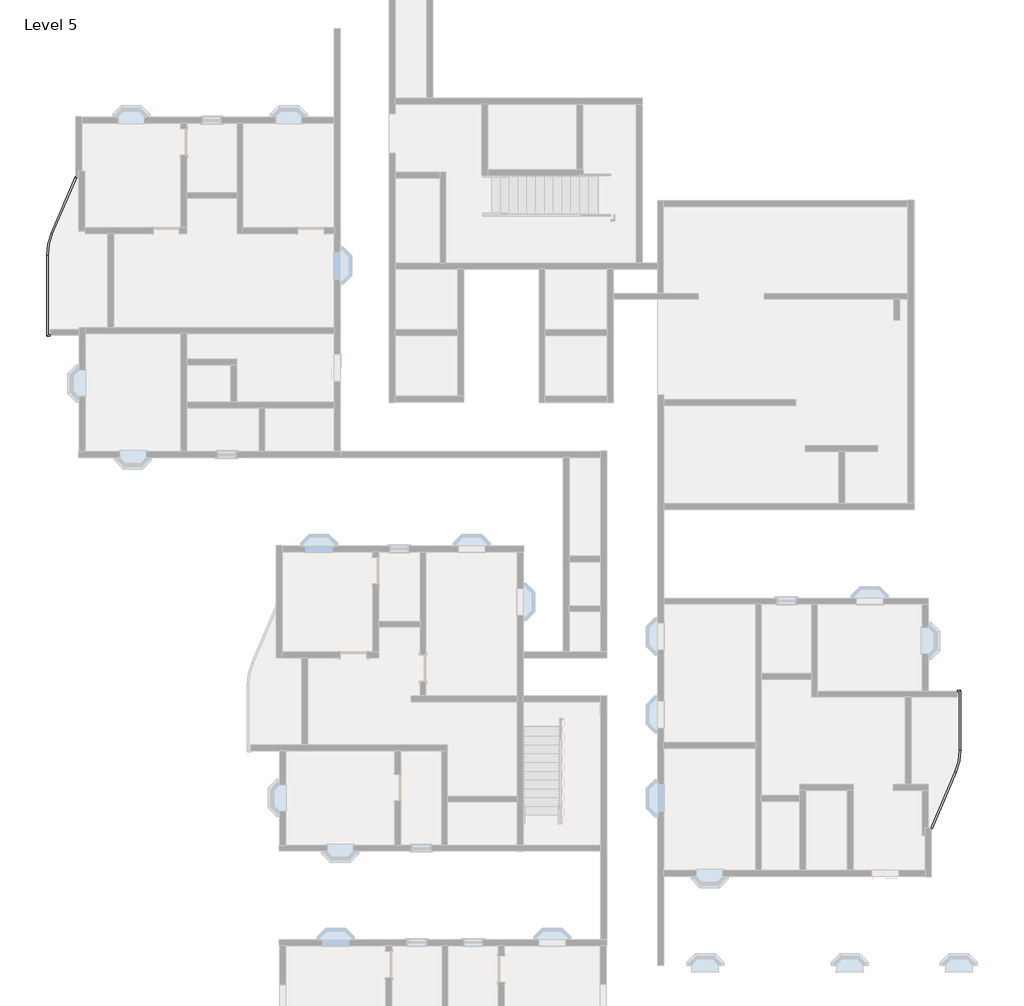
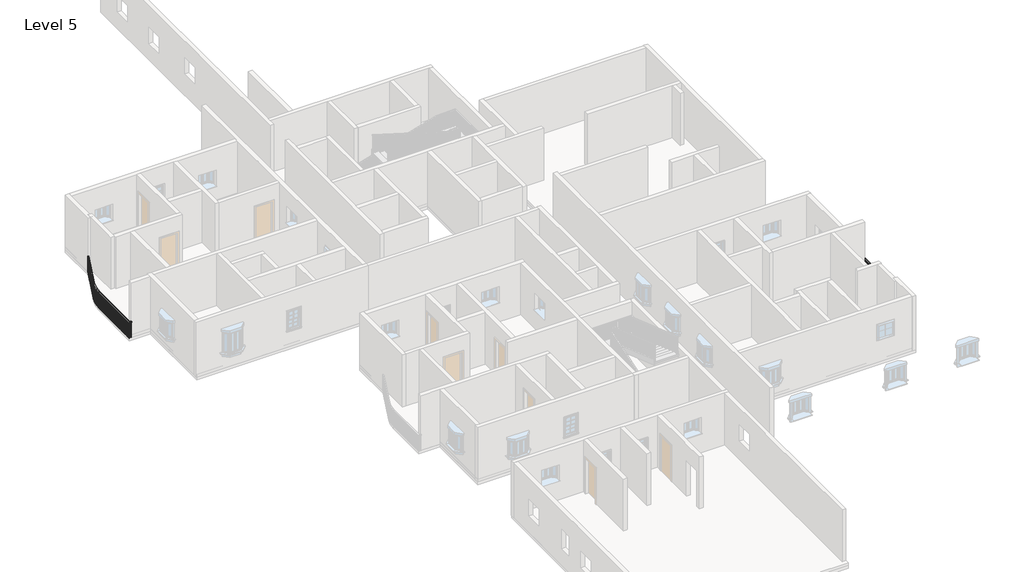
# One storey, part 9 of 14: 2 railings.
"""IFC4 building model written with IfcOpenShell, lengths in millimetres."""

from ifc_helpers import new_model, si_unit, frame, origin, place, context, project, spatial, polyline, circle_curve, outline, extrude, element, save
from ifc_brep_helpers import plane_surface, cylinder_surface, revolved_surface, advanced_brep

model = new_model("IFC4")

# Units and contexts
model_context = context("Model", 3, world=origin())
ifc_project = project(units=[si_unit("LENGTHUNIT", "METRE", prefix="MILLI")], contexts=[model_context])

# Site, building, storey
site = spatial("IfcSite", under=ifc_project)
building = spatial("IfcBuilding", under=site)
storey = spatial("IfcBuildingStorey", under=building, Name="Level 5", Elevation=12192.0)

# Railings
placement = place(None, origin())
element("IfcRailing", 1, ObjectType="Handrail - Rectangular", at=placement, inside=storey, context=model_context, shape_type="SolidModel", body=[
    advanced_brep(
    [(-19327.739878, 12446.0257339, 13106.4), (-19327.739878, 12446.0257339, 13055.6), (-19374.4383922, 12466.022953, 13055.6), (-19374.4383922, 12466.022953, 13106.4), (-20162.483418, 10496.6905323, 13106.4), (-20162.483418, 10496.6905323, 13055.6), (-20209.1819322, 10516.6877514, 13055.6), (-20209.1819322, 10516.6877514, 13106.4), (-20316.2891351, 9746.7948172, 13055.6), (-20316.2891351, 9746.7948172, 13106.4), (-20367.0891351, 9746.7948172, 13055.6), (-20367.0891351, 9746.7948172, 13106.4), (-20316.2891351, 7005.2583494, 13106.4), (-20316.2891351, 7005.2583494, 13055.6), (-20367.0891351, 6954.4583494, 13055.6), (-20367.0891351, 6954.4583494, 13106.4), (-20240.0891351, 7005.2583494, 13106.4), (-20240.0891351, 6954.4583494, 13106.4), (-20240.0891351, 6954.4583494, 13055.6), (-20240.0891351, 7005.2583494, 13055.6)],
    [
        (0, 1),
        (1, 2),
        (2, 3),
        (3, 0),
        (0, 4),
        (4, 5),
        (5, 1),
        (5, 6),
        (6, 2),
        (6, 7),
        (7, 3),
        (7, 4),
        (8, 5, circle_curve(frame((-18411.2891351, 9746.7948172, 13055.6), z_axis=(0.0, 0.0, -1.0), x_axis=(-0.919262090762392, 0.3936460446735823, 0.0)), 1905.0)),
        (4, 9, circle_curve(frame((-18411.2891351, 9746.7948172, 13106.4), z_axis=(0.0, 0.0, 1.0), x_axis=(-0.919262090762392, 0.3936460446735823, 0.0)), 1905.0)),
        (9, 8),
        (10, 6, circle_curve(frame((-18411.2891351, 9746.7948172, 13055.6), z_axis=(0.0, 0.0, -1.0), x_axis=(-0.919262090762392, 0.3936460446735823, 0.0)), 1955.8)),
        (8, 10),
        (11, 7, circle_curve(frame((-18411.2891351, 9746.7948172, 13106.4), z_axis=(0.0, 0.0, -1.0), x_axis=(-0.919262090762392, 0.3936460446735823, 0.0)), 1955.8)),
        (10, 11),
        (11, 9),
        (9, 12),
        (12, 13),
        (13, 8),
        (13, 14),
        (14, 10),
        (14, 15),
        (15, 11),
        (15, 12),
        (16, 17),
        (17, 18),
        (18, 19),
        (19, 16),
        (12, 16),
        (19, 13),
        (18, 14),
        (17, 15),
    ],
    [
        plane_surface(frame((-19351.0891351, 12456.0243434, 13106.4), z_axis=(0.3936460446735829, 0.9192620907623917, 0.0), x_axis=(0.9192620907623917, -0.3936460446735829, 0.0))),
        plane_surface(frame((-19327.739878, 12446.0257339, 13106.4), z_axis=(0.9192620907623915, -0.3936460446735834, 0.0), x_axis=(-0.3936460446735834, -0.9192620907623915, 0.0))),
        plane_surface(frame((-19327.739878, 12446.0257339, 13055.6), z_axis=(0.0, 0.0, -1.0000000000000002), x_axis=(-0.3936460446735834, -0.9192620907623915, 0.0))),
        plane_surface(frame((-19374.4383922, 12466.022953, 13055.6), z_axis=(-0.9192620907623916, 0.393646044673583, 0.0), x_axis=(-0.393646044673583, -0.9192620907623916, 0.0))),
        plane_surface(frame((-19374.4383922, 12466.022953, 13106.4), z_axis=(0.0, 0.0, 1.0), x_axis=(-0.393646044673583, -0.9192620907623916, 0.0))),
        revolved_surface(polyline([(-20162.483418002357, 10496.690532303173, 13106.4), (-20162.483418002357, 10496.690532303173, 13055.6)]), (-18411.2891351, 9746.7948172, 13106.4), (0.0, 0.0, 1.0)),
        plane_surface(frame((-18411.2891351, 9746.7948172, 13055.6), z_axis=(0.0, 0.0, -1.0), x_axis=(-0.919262090762392, 0.3936460446735823, 0.0))),
        cylinder_surface(frame((-18411.2891351, 9746.7948172, 13106.4), z_axis=(0.0, 0.0, 1.0), x_axis=(-0.919262090762392, 0.3936460446735823, 0.0)), 1955.8),
        plane_surface(frame((-18411.2891351, 9746.7948172, 13106.4), z_axis=(0.0, 0.0, 1.0), x_axis=(-0.919262090762392, 0.3936460446735823, 0.0))),
        plane_surface(frame((-20316.2891351, 9746.7948172, 13106.4), z_axis=(1.0, 0.0, 0.0), x_axis=(0.0, -1.0, 0.0))),
        plane_surface(frame((-20316.2891351, 9746.7948172, 13055.6), z_axis=(0.0, 0.0, -1.0), x_axis=(0.0, -1.0, 0.0))),
        plane_surface(frame((-20367.0891351, 9746.7948172, 13055.6), z_axis=(-1.0, 0.0, 0.0), x_axis=(0.0, -1.0, 0.0))),
        plane_surface(frame((-20367.0891351, 9746.7948172, 13106.4), z_axis=(0.0, 0.0, 1.0), x_axis=(0.0, -1.0, 0.0))),
        plane_surface(frame((-20240.0891351, 6979.8583494, 13106.4), z_axis=(1.0, 0.0, 0.0), x_axis=(0.0, 1.0, 0.0))),
        plane_surface(frame((-20316.2891351, 7005.2583494, 13106.4), z_axis=(0.0, 1.0, 0.0), x_axis=(1.0, 0.0, 0.0))),
        plane_surface(frame((-20316.2891351, 7005.2583494, 13055.6), z_axis=(0.0, 0.0, -1.0), x_axis=(1.0, 0.0, 0.0))),
        plane_surface(frame((-20367.0891351, 6954.4583494, 13055.6), z_axis=(0.0, -1.0, 0.0), x_axis=(1.0, 0.0, 0.0))),
        plane_surface(frame((-20367.0891351, 6954.4583494, 13106.4), z_axis=(0.0, 0.0, 1.0), x_axis=(1.0, 0.0, 0.0))),
    ],
    [
        (0, [[1, 2, 3, 4]]),
        (1, [[-1, 5, 6, 7]]),
        (2, [[-2, -7, 8, 9]]),
        (3, [[-3, -9, 10, 11]]),
        (4, [[-4, -11, 12, -5]]),
        (5, [[13, -6, 14, 15]]),
        (6, [[16, -8, -13, 17]]),
        (7, [[18, -10, -16, 19]]),
        (8, [[-14, -12, -18, 20]]),
        (9, [[-15, 21, 22, 23]]),
        (10, [[-17, -23, 24, 25]]),
        (11, [[-19, -25, 26, 27]]),
        (12, [[-20, -27, 28, -21]]),
        (13, [[29, 30, 31, 32]]),
        (14, [[-22, 33, -32, 34]]),
        (15, [[-24, -34, -31, 35]]),
        (16, [[-26, -35, -30, 36]]),
        (17, [[-28, -36, -29, -33]]),
    ],
),
    extrude(outline(polyline([(-20351.2141351, 7013.1198172), (-20332.1641351, 7013.1198172), (-20332.1641351, 6994.0698172), (-20351.2141351, 6994.0698172), (-20351.2141351, 7013.1198172)])), frame((0.0, 0.0, 12192.0), z_axis=(0.0, 0.0, 1.0), x_axis=(1.0, 0.0, 0.0)), (0.0, 0.0, 1.0), 863.6),
    extrude(outline(polyline([(-20351.2141351, 7114.7198172), (-20332.1641351, 7114.7198172), (-20332.1641351, 7095.6698172), (-20351.2141351, 7095.6698172), (-20351.2141351, 7114.7198172)])), frame((0.0, 0.0, 12192.0), z_axis=(0.0, 0.0, 1.0), x_axis=(1.0, 0.0, 0.0)), (0.0, 0.0, 1.0), 863.6),
    extrude(outline(polyline([(-20351.2141351, 7216.3198172), (-20332.1641351, 7216.3198172), (-20332.1641351, 7197.2698172), (-20351.2141351, 7197.2698172), (-20351.2141351, 7216.3198172)])), frame((0.0, 0.0, 12192.0), z_axis=(0.0, 0.0, 1.0), x_axis=(1.0, 0.0, 0.0)), (0.0, 0.0, 1.0), 863.6),
    extrude(outline(polyline([(-20351.2141351, 7317.9198172), (-20332.1641351, 7317.9198172), (-20332.1641351, 7298.8698172), (-20351.2141351, 7298.8698172), (-20351.2141351, 7317.9198172)])), frame((0.0, 0.0, 12192.0), z_axis=(0.0, 0.0, 1.0), x_axis=(1.0, 0.0, 0.0)), (0.0, 0.0, 1.0), 863.6),
    extrude(outline(polyline([(-20351.2141351, 7419.5198172), (-20332.1641351, 7419.5198172), (-20332.1641351, 7400.4698172), (-20351.2141351, 7400.4698172), (-20351.2141351, 7419.5198172)])), frame((0.0, 0.0, 12192.0), z_axis=(0.0, 0.0, 1.0), x_axis=(1.0, 0.0, 0.0)), (0.0, 0.0, 1.0), 863.6),
    extrude(outline(polyline([(-20351.2141351, 7521.1198172), (-20332.1641351, 7521.1198172), (-20332.1641351, 7502.0698172), (-20351.2141351, 7502.0698172), (-20351.2141351, 7521.1198172)])), frame((0.0, 0.0, 12192.0), z_axis=(0.0, 0.0, 1.0), x_axis=(1.0, 0.0, 0.0)), (0.0, 0.0, 1.0), 863.6),
    extrude(outline(polyline([(-20351.2141351, 7622.7198172), (-20332.1641351, 7622.7198172), (-20332.1641351, 7603.6698172), (-20351.2141351, 7603.6698172), (-20351.2141351, 7622.7198172)])), frame((0.0, 0.0, 12192.0), z_axis=(0.0, 0.0, 1.0), x_axis=(1.0, 0.0, 0.0)), (0.0, 0.0, 1.0), 863.6),
    extrude(outline(polyline([(-20351.2141351, 7724.3198172), (-20332.1641351, 7724.3198172), (-20332.1641351, 7705.2698172), (-20351.2141351, 7705.2698172), (-20351.2141351, 7724.3198172)])), frame((0.0, 0.0, 12192.0), z_axis=(0.0, 0.0, 1.0), x_axis=(1.0, 0.0, 0.0)), (0.0, 0.0, 1.0), 863.6),
    extrude(outline(polyline([(-20351.2141351, 7825.9198172), (-20332.1641351, 7825.9198172), (-20332.1641351, 7806.8698172), (-20351.2141351, 7806.8698172), (-20351.2141351, 7825.9198172)])), frame((0.0, 0.0, 12192.0), z_axis=(0.0, 0.0, 1.0), x_axis=(1.0, 0.0, 0.0)), (0.0, 0.0, 1.0), 863.6),
    extrude(outline(polyline([(-20351.2141351, 7927.5198172), (-20332.1641351, 7927.5198172), (-20332.1641351, 7908.4698172), (-20351.2141351, 7908.4698172), (-20351.2141351, 7927.5198172)])), frame((0.0, 0.0, 12192.0), z_axis=(0.0, 0.0, 1.0), x_axis=(1.0, 0.0, 0.0)), (0.0, 0.0, 1.0), 863.6),
    extrude(outline(polyline([(-20351.2141351, 8029.1198172), (-20332.1641351, 8029.1198172), (-20332.1641351, 8010.0698172), (-20351.2141351, 8010.0698172), (-20351.2141351, 8029.1198172)])), frame((0.0, 0.0, 12192.0), z_axis=(0.0, 0.0, 1.0), x_axis=(1.0, 0.0, 0.0)), (0.0, 0.0, 1.0), 863.6),
    extrude(outline(polyline([(-20351.2141351, 8130.7198172), (-20332.1641351, 8130.7198172), (-20332.1641351, 8111.6698172), (-20351.2141351, 8111.6698172), (-20351.2141351, 8130.7198172)])), frame((0.0, 0.0, 12192.0), z_axis=(0.0, 0.0, 1.0), x_axis=(1.0, 0.0, 0.0)), (0.0, 0.0, 1.0), 863.6),
    extrude(outline(polyline([(-20351.2141351, 8232.3198172), (-20332.1641351, 8232.3198172), (-20332.1641351, 8213.2698172), (-20351.2141351, 8213.2698172), (-20351.2141351, 8232.3198172)])), frame((0.0, 0.0, 12192.0), z_axis=(0.0, 0.0, 1.0), x_axis=(1.0, 0.0, 0.0)), (0.0, 0.0, 1.0), 863.6),
    extrude(outline(polyline([(-20351.2141351, 8333.9198172), (-20332.1641351, 8333.9198172), (-20332.1641351, 8314.8698172), (-20351.2141351, 8314.8698172), (-20351.2141351, 8333.9198172)])), frame((0.0, 0.0, 12192.0), z_axis=(0.0, 0.0, 1.0), x_axis=(1.0, 0.0, 0.0)), (0.0, 0.0, 1.0), 863.6),
    extrude(outline(polyline([(-20351.2141351, 8435.5198172), (-20332.1641351, 8435.5198172), (-20332.1641351, 8416.4698172), (-20351.2141351, 8416.4698172), (-20351.2141351, 8435.5198172)])), frame((0.0, 0.0, 12192.0), z_axis=(0.0, 0.0, 1.0), x_axis=(1.0, 0.0, 0.0)), (0.0, 0.0, 1.0), 863.6),
    extrude(outline(polyline([(-20351.2141351, 8537.1198172), (-20332.1641351, 8537.1198172), (-20332.1641351, 8518.0698172), (-20351.2141351, 8518.0698172), (-20351.2141351, 8537.1198172)])), frame((0.0, 0.0, 12192.0), z_axis=(0.0, 0.0, 1.0), x_axis=(1.0, 0.0, 0.0)), (0.0, 0.0, 1.0), 863.6),
    extrude(outline(polyline([(-20351.2141351, 8638.7198172), (-20332.1641351, 8638.7198172), (-20332.1641351, 8619.6698172), (-20351.2141351, 8619.6698172), (-20351.2141351, 8638.7198172)])), frame((0.0, 0.0, 12192.0), z_axis=(0.0, 0.0, 1.0), x_axis=(1.0, 0.0, 0.0)), (0.0, 0.0, 1.0), 863.6),
    extrude(outline(polyline([(-20351.2141351, 8740.3198172), (-20332.1641351, 8740.3198172), (-20332.1641351, 8721.2698172), (-20351.2141351, 8721.2698172), (-20351.2141351, 8740.3198172)])), frame((0.0, 0.0, 12192.0), z_axis=(0.0, 0.0, 1.0), x_axis=(1.0, 0.0, 0.0)), (0.0, 0.0, 1.0), 863.6),
    extrude(outline(polyline([(-20351.2141351, 8841.9198172), (-20332.1641351, 8841.9198172), (-20332.1641351, 8822.8698172), (-20351.2141351, 8822.8698172), (-20351.2141351, 8841.9198172)])), frame((0.0, 0.0, 12192.0), z_axis=(0.0, 0.0, 1.0), x_axis=(1.0, 0.0, 0.0)), (0.0, 0.0, 1.0), 863.6),
    extrude(outline(polyline([(-20351.2141351, 8943.5198172), (-20332.1641351, 8943.5198172), (-20332.1641351, 8924.4698172), (-20351.2141351, 8924.4698172), (-20351.2141351, 8943.5198172)])), frame((0.0, 0.0, 12192.0), z_axis=(0.0, 0.0, 1.0), x_axis=(1.0, 0.0, 0.0)), (0.0, 0.0, 1.0), 863.6),
    extrude(outline(polyline([(-20351.2141351, 9045.1198172), (-20332.1641351, 9045.1198172), (-20332.1641351, 9026.0698172), (-20351.2141351, 9026.0698172), (-20351.2141351, 9045.1198172)])), frame((0.0, 0.0, 12192.0), z_axis=(0.0, 0.0, 1.0), x_axis=(1.0, 0.0, 0.0)), (0.0, 0.0, 1.0), 863.6),
    extrude(outline(polyline([(-20351.2141351, 9146.7198172), (-20332.1641351, 9146.7198172), (-20332.1641351, 9127.6698172), (-20351.2141351, 9127.6698172), (-20351.2141351, 9146.7198172)])), frame((0.0, 0.0, 12192.0), z_axis=(0.0, 0.0, 1.0), x_axis=(1.0, 0.0, 0.0)), (0.0, 0.0, 1.0), 863.6),
    extrude(outline(polyline([(-20351.2141351, 9248.3198172), (-20332.1641351, 9248.3198172), (-20332.1641351, 9229.2698172), (-20351.2141351, 9229.2698172), (-20351.2141351, 9248.3198172)])), frame((0.0, 0.0, 12192.0), z_axis=(0.0, 0.0, 1.0), x_axis=(1.0, 0.0, 0.0)), (0.0, 0.0, 1.0), 863.6),
    extrude(outline(polyline([(-20351.2141351, 9349.9198172), (-20332.1641351, 9349.9198172), (-20332.1641351, 9330.8698172), (-20351.2141351, 9330.8698172), (-20351.2141351, 9349.9198172)])), frame((0.0, 0.0, 12192.0), z_axis=(0.0, 0.0, 1.0), x_axis=(1.0, 0.0, 0.0)), (0.0, 0.0, 1.0), 863.6),
    extrude(outline(polyline([(-20351.2141351, 9451.5198172), (-20332.1641351, 9451.5198172), (-20332.1641351, 9432.4698172), (-20351.2141351, 9432.4698172), (-20351.2141351, 9451.5198172)])), frame((0.0, 0.0, 12192.0), z_axis=(0.0, 0.0, 1.0), x_axis=(1.0, 0.0, 0.0)), (0.0, 0.0, 1.0), 863.6),
    extrude(outline(polyline([(-20351.2141351, 9553.1198172), (-20332.1641351, 9553.1198172), (-20332.1641351, 9534.0698172), (-20351.2141351, 9534.0698172), (-20351.2141351, 9553.1198172)])), frame((0.0, 0.0, 12192.0), z_axis=(0.0, 0.0, 1.0), x_axis=(1.0, 0.0, 0.0)), (0.0, 0.0, 1.0), 863.6),
    extrude(outline(polyline([(-20351.2141351, 9654.7198172), (-20332.1641351, 9654.7198172), (-20332.1641351, 9635.6698172), (-20351.2141351, 9635.6698172), (-20351.2141351, 9654.7198172)])), frame((0.0, 0.0, 12192.0), z_axis=(0.0, 0.0, 1.0), x_axis=(1.0, 0.0, 0.0)), (0.0, 0.0, 1.0), 863.6),
    extrude(outline(polyline([(-20349.6005818, 9826.4720848), (-20330.5630441, 9825.7831307), (-20331.2519982, 9806.745593), (-20350.289536, 9807.4345471), (-20349.6005818, 9826.4720848)])), frame((0.0, 0.0, 12192.0), z_axis=(0.0, 0.0, 1.0), x_axis=(1.0, 0.0, 0.0)), (0.0, 0.0, 1.0), 863.6),
    extrude(outline(polyline([(-20342.724955, 9928.3310534), (-20323.750023, 9926.6415402), (-20325.4395363, 9907.6666081), (-20344.4144683, 9909.3561214), (-20342.724955, 9928.3310534)])), frame((0.0, 0.0, 12192.0), z_axis=(0.0, 0.0, 1.0), x_axis=(1.0, 0.0, 0.0)), (0.0, 0.0, 1.0), 863.6),
    extrude(outline(polyline([(-20330.5003254, 10029.6872677), (-20311.6405491, 10027.0018743), (-20314.3259425, 10008.142098), (-20333.1857188, 10010.8274914), (-20330.5003254, 10029.6872677)])), frame((0.0, 0.0, 12192.0), z_axis=(0.0, 0.0, 1.0), x_axis=(1.0, 0.0, 0.0)), (0.0, 0.0, 1.0), 863.6),
    extrude(outline(polyline([(-20312.9605484, 10130.2600272), (-20294.2681589, 10126.5861907), (-20297.9419954, 10107.8938012), (-20316.6343849, 10111.5676377), (-20312.9605484, 10130.2600272)])), frame((0.0, 0.0, 12192.0), z_axis=(0.0, 0.0, 1.0), x_axis=(1.0, 0.0, 0.0)), (0.0, 0.0, 1.0), 863.6),
    extrude(outline(polyline([(-20290.1541995, 10229.7708014), (-20271.6809643, 10225.1186963), (-20276.3330693, 10206.6454611), (-20294.8063045, 10211.2975662), (-20290.1541995, 10229.7708014)])), frame((0.0, 0.0, 12192.0), z_axis=(0.0, 0.0, 1.0), x_axis=(1.0, 0.0, 0.0)), (0.0, 0.0, 1.0), 863.6),
    extrude(outline(polyline([(-20262.1444395, 10327.9440008), (-20243.9415192, 10322.3265109), (-20249.5590091, 10304.1235906), (-20267.7619294, 10309.7410805), (-20262.1444395, 10327.9440008)])), frame((0.0, 0.0, 12192.0), z_axis=(0.0, 0.0, 1.0), x_axis=(1.0, 0.0, 0.0)), (0.0, 0.0, 1.0), 863.6),
    extrude(outline(polyline([(-20229.0088399, 10424.5077402), (-20211.1266465, 10417.9404228), (-20217.693964, 10400.0582293), (-20235.5761574, 10406.6255468), (-20229.0088399, 10424.5077402)])), frame((0.0, 0.0, 12192.0), z_axis=(0.0, 0.0, 1.0), x_axis=(1.0, 0.0, 0.0)), (0.0, 0.0, 1.0), 863.6),
    extrude(outline(polyline([(-20155.9843907, 10600.589225), (-20138.4724479, 10593.0902678), (-20145.9714051, 10575.578325), (-20163.4833479, 10583.0772822), (-20155.9843907, 10600.589225)])), frame((0.0, 0.0, 12192.0), z_axis=(0.0, 0.0, 1.0), x_axis=(1.0, 0.0, 0.0)), (0.0, 0.0, 1.0), 863.6),
    extrude(outline(polyline([(-20115.9899526, 10693.9862534), (-20098.4780098, 10686.4872963), (-20105.9769669, 10668.9753534), (-20123.4889098, 10676.4743106), (-20115.9899526, 10693.9862534)])), frame((0.0, 0.0, 12192.0), z_axis=(0.0, 0.0, 1.0), x_axis=(1.0, 0.0, 0.0)), (0.0, 0.0, 1.0), 863.6),
    extrude(outline(polyline([(-20075.9955145, 10787.3832818), (-20058.4835716, 10779.8843247), (-20065.9825288, 10762.3723818), (-20083.4944716, 10769.871339), (-20075.9955145, 10787.3832818)])), frame((0.0, 0.0, 12192.0), z_axis=(0.0, 0.0, 1.0), x_axis=(1.0, 0.0, 0.0)), (0.0, 0.0, 1.0), 863.6),
    extrude(outline(polyline([(-20036.0010763, 10880.7803103), (-20018.4891335, 10873.2813531), (-20025.9880906, 10855.7694103), (-20043.5000335, 10863.2683674), (-20036.0010763, 10880.7803103)])), frame((0.0, 0.0, 12192.0), z_axis=(0.0, 0.0, 1.0), x_axis=(1.0, 0.0, 0.0)), (0.0, 0.0, 1.0), 863.6),
    extrude(outline(polyline([(-19996.0066382, 10974.1773387), (-19978.4946954, 10966.6783815), (-19985.9936525, 10949.1664387), (-20003.5055953, 10956.6653958), (-19996.0066382, 10974.1773387)])), frame((0.0, 0.0, 12192.0), z_axis=(0.0, 0.0, 1.0), x_axis=(1.0, 0.0, 0.0)), (0.0, 0.0, 1.0), 863.6),
    extrude(outline(polyline([(-19956.0122, 11067.5743671), (-19938.5002572, 11060.0754099), (-19945.9992144, 11042.5634671), (-19963.5111572, 11050.0624243), (-19956.0122, 11067.5743671)])), frame((0.0, 0.0, 12192.0), z_axis=(0.0, 0.0, 1.0), x_axis=(1.0, 0.0, 0.0)), (0.0, 0.0, 1.0), 863.6),
    extrude(outline(polyline([(-19916.0177619, 11160.9713955), (-19898.5058191, 11153.4724384), (-19906.0047762, 11135.9604955), (-19923.5167191, 11143.4594527), (-19916.0177619, 11160.9713955)])), frame((0.0, 0.0, 12192.0), z_axis=(0.0, 0.0, 1.0), x_axis=(1.0, 0.0, 0.0)), (0.0, 0.0, 1.0), 863.6),
    extrude(outline(polyline([(-19876.0233238, 11254.3684239), (-19858.5113809, 11246.8694668), (-19866.0103381, 11229.357524), (-19883.5222809, 11236.8564811), (-19876.0233238, 11254.3684239)])), frame((0.0, 0.0, 12192.0), z_axis=(0.0, 0.0, 1.0), x_axis=(1.0, 0.0, 0.0)), (0.0, 0.0, 1.0), 863.6),
    extrude(outline(polyline([(-19836.0288856, 11347.7654524), (-19818.5169428, 11340.2664952), (-19826.0159, 11322.7545524), (-19843.5278428, 11330.2535095), (-19836.0288856, 11347.7654524)])), frame((0.0, 0.0, 12192.0), z_axis=(0.0, 0.0, 1.0), x_axis=(1.0, 0.0, 0.0)), (0.0, 0.0, 1.0), 863.6),
    extrude(outline(polyline([(-19796.0344475, 11441.1624808), (-19778.5225047, 11433.6635236), (-19786.0214618, 11416.1515808), (-19803.5334046, 11423.650538), (-19796.0344475, 11441.1624808)])), frame((0.0, 0.0, 12192.0), z_axis=(0.0, 0.0, 1.0), x_axis=(1.0, 0.0, 0.0)), (0.0, 0.0, 1.0), 863.6),
    extrude(outline(polyline([(-19756.0400094, 11534.5595092), (-19738.5280665, 11527.060552), (-19746.0270237, 11509.5486092), (-19763.5389665, 11517.0475664), (-19756.0400094, 11534.5595092)])), frame((0.0, 0.0, 12192.0), z_axis=(0.0, 0.0, 1.0), x_axis=(1.0, 0.0, 0.0)), (0.0, 0.0, 1.0), 863.6),
    extrude(outline(polyline([(-19716.0455712, 11627.9565376), (-19698.5336284, 11620.4575805), (-19706.0325855, 11602.9456376), (-19723.5445284, 11610.4445948), (-19716.0455712, 11627.9565376)])), frame((0.0, 0.0, 12192.0), z_axis=(0.0, 0.0, 1.0), x_axis=(1.0, 0.0, 0.0)), (0.0, 0.0, 1.0), 863.6),
    extrude(outline(polyline([(-19676.0511331, 11721.353566), (-19658.5391902, 11713.8546089), (-19666.0381474, 11696.3426661), (-19683.5500902, 11703.8416232), (-19676.0511331, 11721.353566)])), frame((0.0, 0.0, 12192.0), z_axis=(0.0, 0.0, 1.0), x_axis=(1.0, 0.0, 0.0)), (0.0, 0.0, 1.0), 863.6),
    extrude(outline(polyline([(-19636.0566949, 11814.7505945), (-19618.5447521, 11807.2516373), (-19626.0437093, 11789.7396945), (-19643.5556521, 11797.2386516), (-19636.0566949, 11814.7505945)])), frame((0.0, 0.0, 12192.0), z_axis=(0.0, 0.0, 1.0), x_axis=(1.0, 0.0, 0.0)), (0.0, 0.0, 1.0), 863.6),
    extrude(outline(polyline([(-19596.0622568, 11908.1476229), (-19578.550314, 11900.6486657), (-19586.0492711, 11883.1367229), (-19603.561214, 11890.6356801), (-19596.0622568, 11908.1476229)])), frame((0.0, 0.0, 12192.0), z_axis=(0.0, 0.0, 1.0), x_axis=(1.0, 0.0, 0.0)), (0.0, 0.0, 1.0), 863.6),
    extrude(outline(polyline([(-19556.0678187, 12001.5446513), (-19538.5558758, 11994.0456942), (-19546.054833, 11976.5337513), (-19563.5667758, 11984.0327085), (-19556.0678187, 12001.5446513)])), frame((0.0, 0.0, 12192.0), z_axis=(0.0, 0.0, 1.0), x_axis=(1.0, 0.0, 0.0)), (0.0, 0.0, 1.0), 863.6),
    extrude(outline(polyline([(-19516.0733805, 12094.9416797), (-19498.5614377, 12087.4427226), (-19506.0603948, 12069.9307797), (-19523.5723377, 12077.4297369), (-19516.0733805, 12094.9416797)])), frame((0.0, 0.0, 12192.0), z_axis=(0.0, 0.0, 1.0), x_axis=(1.0, 0.0, 0.0)), (0.0, 0.0, 1.0), 863.6),
    extrude(outline(polyline([(-19476.0789424, 12188.3387082), (-19458.5669996, 12180.839751), (-19466.0659567, 12163.3278082), (-19483.5778995, 12170.8267653), (-19476.0789424, 12188.3387082)])), frame((0.0, 0.0, 12192.0), z_axis=(0.0, 0.0, 1.0), x_axis=(1.0, 0.0, 0.0)), (0.0, 0.0, 1.0), 863.6),
    extrude(outline(polyline([(-19436.0845042, 12281.7357366), (-19418.5725614, 12274.2367794), (-19426.0715186, 12256.7248366), (-19443.5834614, 12264.2237937), (-19436.0845042, 12281.7357366)])), frame((0.0, 0.0, 12192.0), z_axis=(0.0, 0.0, 1.0), x_axis=(1.0, 0.0, 0.0)), (0.0, 0.0, 1.0), 863.6),
    extrude(outline(polyline([(-19396.0900661, 12375.132765), (-19378.5781233, 12367.6338078), (-19386.0770804, 12350.121865), (-19403.5890233, 12357.6208222), (-19396.0900661, 12375.132765)])), frame((0.0, 0.0, 12192.0), z_axis=(0.0, 0.0, 1.0), x_axis=(1.0, 0.0, 0.0)), (0.0, 0.0, 1.0), 863.6),
    extrude(outline(polyline([(-20351.2141351, 6989.3833494), (-20332.1641351, 6989.3833494), (-20332.1641351, 6970.3333494), (-20351.2141351, 6970.3333494), (-20351.2141351, 6989.3833494)])), frame((0.0, 0.0, 12192.0), z_axis=(0.0, 0.0, 1.0), x_axis=(1.0, 0.0, 0.0)), (0.0, 0.0, 1.0), 863.6),
    extrude(outline(polyline([(-20351.2141351, 9756.3198172), (-20332.1641351, 9756.3198172), (-20332.1641351, 9737.2698172), (-20351.2141351, 9737.2698172), (-20351.2141351, 9756.3198172)])), frame((0.0, 0.0, 12192.0), z_axis=(0.0, 0.0, 1.0), x_axis=(1.0, 0.0, 0.0)), (0.0, 0.0, 1.0), 863.6),
    extrude(outline(polyline([(-20190.839168, 10519.1945919), (-20173.3272251, 10511.6956347), (-20180.8261823, 10494.1836919), (-20198.3381251, 10501.682649), (-20190.839168, 10519.1945919)])), frame((0.0, 0.0, 12192.0), z_axis=(0.0, 0.0, 1.0), x_axis=(1.0, 0.0, 0.0)), (0.0, 0.0, 1.0), 863.6),
    extrude(outline(polyline([(-20259.1391351, 6970.3333494), (-20259.1391351, 6989.3833494), (-20240.0891351, 6989.3833494), (-20240.0891351, 6970.3333494), (-20259.1391351, 6970.3333494)])), frame((0.0, 0.0, 12192.0), z_axis=(0.0, 0.0, 1.0), x_axis=(1.0, 0.0, 0.0)), (0.0, 0.0, 1.0), 863.6),
    extrude(outline(polyline([(-19359.8451065, 12459.773822), (-19342.3331637, 12452.2748648), (-19349.8321209, 12434.762922), (-19367.3440637, 12442.2618792), (-19359.8451065, 12459.773822)])), frame((0.0, 0.0, 12192.0), z_axis=(0.0, 0.0, 1.0), x_axis=(1.0, 0.0, 0.0)), (0.0, 0.0, 1.0), 863.6),
])
element("IfcRailing", 2, ObjectType="Handrail - Rectangular", at=placement, inside=storey, context=model_context, shape_type="SolidModel", body=[
    advanced_brep(
    [(10250.7887952, -10096.81198, 13106.4), (10250.7887952, -10096.81198, 13055.6), (10297.4873094, -10116.8091991, 13055.6), (10297.4873094, -10116.8091991, 13106.4), (11085.5323352, -8147.4767784, 13106.4), (11085.5323352, -8147.4767784, 13055.6), (11132.2308494, -8167.4739975, 13055.6), (11132.2308494, -8167.4739975, 13106.4), (11239.3380523, -7397.5810633, 13055.6), (11239.3380523, -7397.5810633, 13106.4), (11290.1380523, -7397.5810633, 13055.6), (11290.1380523, -7397.5810633, 13106.4), (11239.3380523, -5378.0542694, 13106.4), (11239.3380523, -5378.0542694, 13055.6), (11290.1380523, -5327.2542694, 13055.6), (11290.1380523, -5327.2542694, 13106.4), (11163.1380523, -5378.0542694, 13106.4), (11163.1380523, -5327.2542694, 13106.4), (11163.1380523, -5327.2542694, 13055.6), (11163.1380523, -5378.0542694, 13055.6)],
    [
        (0, 1),
        (1, 2),
        (2, 3),
        (3, 0),
        (0, 4),
        (4, 5),
        (5, 1),
        (5, 6),
        (6, 2),
        (6, 7),
        (7, 3),
        (7, 4),
        (8, 5, circle_curve(frame((9334.3380523, -7397.5810633, 13055.6), z_axis=(0.0, 0.0, -1.0), x_axis=(0.9192620907624003, -0.3936460446735628, 0.0)), 1905.0)),
        (4, 9, circle_curve(frame((9334.3380523, -7397.5810633, 13106.4), z_axis=(0.0, 0.0, 1.0), x_axis=(0.9192620907624003, -0.3936460446735628, 0.0)), 1905.0)),
        (9, 8),
        (10, 6, circle_curve(frame((9334.3380523, -7397.5810633, 13055.6), z_axis=(0.0, 0.0, -1.0), x_axis=(0.9192620907624003, -0.3936460446735628, 0.0)), 1955.8)),
        (8, 10),
        (11, 7, circle_curve(frame((9334.3380523, -7397.5810633, 13106.4), z_axis=(0.0, 0.0, -1.0), x_axis=(0.9192620907624003, -0.3936460446735628, 0.0)), 1955.8)),
        (10, 11),
        (11, 9),
        (9, 12),
        (12, 13),
        (13, 8),
        (13, 14),
        (14, 10),
        (14, 15),
        (15, 11),
        (15, 12),
        (16, 17),
        (17, 18),
        (18, 19),
        (19, 16),
        (12, 16),
        (19, 13),
        (18, 14),
        (17, 15),
    ],
    [
        plane_surface(frame((10274.1380523, -10106.8105895, 13106.4), z_axis=(-0.3936460446735629, -0.9192620907624003, 0.0), x_axis=(0.9192620907624003, -0.3936460446735629, 0.0))),
        plane_surface(frame((10250.7887952, -10096.81198, 13106.4), z_axis=(-0.9192620907624005, 0.39364604467356235, 0.0), x_axis=(0.39364604467356235, 0.9192620907624005, 0.0))),
        plane_surface(frame((10250.7887952, -10096.81198, 13055.6), z_axis=(0.0, 0.0, -1.0), x_axis=(0.39364604467356235, 0.9192620907624005, 0.0))),
        plane_surface(frame((10297.4873094, -10116.8091991, 13055.6), z_axis=(0.9192620907624003, -0.3936460446735627, 0.0), x_axis=(0.3936460446735627, 0.9192620907624003, 0.0))),
        plane_surface(frame((10297.4873094, -10116.8091991, 13106.4), z_axis=(0.0, 0.0, 1.0), x_axis=(0.3936460446735627, 0.9192620907624003, 0.0))),
        revolved_surface(polyline([(11085.532335202372, -8147.476778403137, 13106.4), (11085.532335202372, -8147.476778403137, 13055.6)]), (9334.3380523, -7397.5810633, 13106.4), (0.0, 0.0, 1.0)),
        plane_surface(frame((9334.3380523, -7397.5810633, 13055.6), z_axis=(0.0, 0.0, -1.0), x_axis=(0.9192620907624003, -0.3936460446735628, 0.0))),
        cylinder_surface(frame((9334.3380523, -7397.5810633, 13106.4), z_axis=(0.0, 0.0, 1.0), x_axis=(0.9192620907624003, -0.3936460446735628, 0.0)), 1955.8),
        plane_surface(frame((9334.3380523, -7397.5810633, 13106.4), z_axis=(0.0, 0.0, 1.0), x_axis=(0.9192620907624003, -0.3936460446735628, 0.0))),
        plane_surface(frame((11239.3380523, -7397.5810633, 13106.4), z_axis=(-1.0, 0.0, 0.0), x_axis=(0.0, 1.0, 0.0))),
        plane_surface(frame((11239.3380523, -7397.5810633, 13055.6), z_axis=(0.0, 0.0, -1.0), x_axis=(0.0, 1.0, 0.0))),
        plane_surface(frame((11290.1380523, -7397.5810633, 13055.6), z_axis=(1.0, 0.0, 0.0), x_axis=(0.0, 1.0, 0.0))),
        plane_surface(frame((11290.1380523, -7397.5810633, 13106.4), z_axis=(0.0, 0.0, 1.0), x_axis=(0.0, 1.0, 0.0))),
        plane_surface(frame((11163.1380523, -5352.6542694, 13106.4), z_axis=(-1.0, 0.0, 0.0), x_axis=(0.0, -1.0, 0.0))),
        plane_surface(frame((11239.3380523, -5378.0542694, 13106.4), z_axis=(0.0, -1.0, 0.0), x_axis=(-1.0, 0.0, 0.0))),
        plane_surface(frame((11239.3380523, -5378.0542694, 13055.6), z_axis=(0.0, 0.0, -1.0), x_axis=(-1.0, 0.0, 0.0))),
        plane_surface(frame((11290.1380523, -5327.2542694, 13055.6), z_axis=(0.0, 1.0, 0.0), x_axis=(-1.0, 0.0, 0.0))),
        plane_surface(frame((11290.1380523, -5327.2542694, 13106.4), z_axis=(0.0, 0.0, 1.0), x_axis=(-1.0, 0.0, 0.0))),
    ],
    [
        (0, [[1, 2, 3, 4]]),
        (1, [[-1, 5, 6, 7]]),
        (2, [[-2, -7, 8, 9]]),
        (3, [[-3, -9, 10, 11]]),
        (4, [[-4, -11, 12, -5]]),
        (5, [[13, -6, 14, 15]]),
        (6, [[16, -8, -13, 17]]),
        (7, [[18, -10, -16, 19]]),
        (8, [[-14, -12, -18, 20]]),
        (9, [[-15, 21, 22, 23]]),
        (10, [[-17, -23, 24, 25]]),
        (11, [[-19, -25, 26, 27]]),
        (12, [[-20, -27, 28, -21]]),
        (13, [[29, 30, 31, 32]]),
        (14, [[-22, 33, -32, 34]]),
        (15, [[-24, -34, -31, 35]]),
        (16, [[-26, -35, -30, 36]]),
        (17, [[-28, -36, -29, -33]]),
    ],
),
    extrude(outline(polyline([(11274.2630523, -5375.1060633), (11255.2130523, -5375.1060633), (11255.2130523, -5356.0560633), (11274.2630523, -5356.0560633), (11274.2630523, -5375.1060633)])), frame((0.0, 0.0, 12192.0), z_axis=(0.0, 0.0, 1.0), x_axis=(1.0, 0.0, 0.0)), (0.0, 0.0, 1.0), 863.6),
    extrude(outline(polyline([(11274.2630523, -5476.7060633), (11255.2130523, -5476.7060633), (11255.2130523, -5457.6560633), (11274.2630523, -5457.6560633), (11274.2630523, -5476.7060633)])), frame((0.0, 0.0, 12192.0), z_axis=(0.0, 0.0, 1.0), x_axis=(1.0, 0.0, 0.0)), (0.0, 0.0, 1.0), 863.6),
    extrude(outline(polyline([(11274.2630523, -5578.3060633), (11255.2130523, -5578.3060633), (11255.2130523, -5559.2560633), (11274.2630523, -5559.2560633), (11274.2630523, -5578.3060633)])), frame((0.0, 0.0, 12192.0), z_axis=(0.0, 0.0, 1.0), x_axis=(1.0, 0.0, 0.0)), (0.0, 0.0, 1.0), 863.6),
    extrude(outline(polyline([(11274.2630523, -5679.9060633), (11255.2130523, -5679.9060633), (11255.2130523, -5660.8560633), (11274.2630523, -5660.8560633), (11274.2630523, -5679.9060633)])), frame((0.0, 0.0, 12192.0), z_axis=(0.0, 0.0, 1.0), x_axis=(1.0, 0.0, 0.0)), (0.0, 0.0, 1.0), 863.6),
    extrude(outline(polyline([(11274.2630523, -5781.5060633), (11255.2130523, -5781.5060633), (11255.2130523, -5762.4560633), (11274.2630523, -5762.4560633), (11274.2630523, -5781.5060633)])), frame((0.0, 0.0, 12192.0), z_axis=(0.0, 0.0, 1.0), x_axis=(1.0, 0.0, 0.0)), (0.0, 0.0, 1.0), 863.6),
    extrude(outline(polyline([(11274.2630523, -5883.1060633), (11255.2130523, -5883.1060633), (11255.2130523, -5864.0560633), (11274.2630523, -5864.0560633), (11274.2630523, -5883.1060633)])), frame((0.0, 0.0, 12192.0), z_axis=(0.0, 0.0, 1.0), x_axis=(1.0, 0.0, 0.0)), (0.0, 0.0, 1.0), 863.6),
    extrude(outline(polyline([(11274.2630523, -5984.7060633), (11255.2130523, -5984.7060633), (11255.2130523, -5965.6560633), (11274.2630523, -5965.6560633), (11274.2630523, -5984.7060633)])), frame((0.0, 0.0, 12192.0), z_axis=(0.0, 0.0, 1.0), x_axis=(1.0, 0.0, 0.0)), (0.0, 0.0, 1.0), 863.6),
    extrude(outline(polyline([(11274.2630523, -6086.3060633), (11255.2130523, -6086.3060633), (11255.2130523, -6067.2560633), (11274.2630523, -6067.2560633), (11274.2630523, -6086.3060633)])), frame((0.0, 0.0, 12192.0), z_axis=(0.0, 0.0, 1.0), x_axis=(1.0, 0.0, 0.0)), (0.0, 0.0, 1.0), 863.6),
    extrude(outline(polyline([(11274.2630523, -6187.9060633), (11255.2130523, -6187.9060633), (11255.2130523, -6168.8560633), (11274.2630523, -6168.8560633), (11274.2630523, -6187.9060633)])), frame((0.0, 0.0, 12192.0), z_axis=(0.0, 0.0, 1.0), x_axis=(1.0, 0.0, 0.0)), (0.0, 0.0, 1.0), 863.6),
    extrude(outline(polyline([(11274.2630523, -6289.5060633), (11255.2130523, -6289.5060633), (11255.2130523, -6270.4560633), (11274.2630523, -6270.4560633), (11274.2630523, -6289.5060633)])), frame((0.0, 0.0, 12192.0), z_axis=(0.0, 0.0, 1.0), x_axis=(1.0, 0.0, 0.0)), (0.0, 0.0, 1.0), 863.6),
    extrude(outline(polyline([(11274.2630523, -6391.1060633), (11255.2130523, -6391.1060633), (11255.2130523, -6372.0560633), (11274.2630523, -6372.0560633), (11274.2630523, -6391.1060633)])), frame((0.0, 0.0, 12192.0), z_axis=(0.0, 0.0, 1.0), x_axis=(1.0, 0.0, 0.0)), (0.0, 0.0, 1.0), 863.6),
    extrude(outline(polyline([(11274.2630523, -6492.7060633), (11255.2130523, -6492.7060633), (11255.2130523, -6473.6560633), (11274.2630523, -6473.6560633), (11274.2630523, -6492.7060633)])), frame((0.0, 0.0, 12192.0), z_axis=(0.0, 0.0, 1.0), x_axis=(1.0, 0.0, 0.0)), (0.0, 0.0, 1.0), 863.6),
    extrude(outline(polyline([(11274.2630523, -6594.3060633), (11255.2130523, -6594.3060633), (11255.2130523, -6575.2560633), (11274.2630523, -6575.2560633), (11274.2630523, -6594.3060633)])), frame((0.0, 0.0, 12192.0), z_axis=(0.0, 0.0, 1.0), x_axis=(1.0, 0.0, 0.0)), (0.0, 0.0, 1.0), 863.6),
    extrude(outline(polyline([(11274.2630523, -6695.9060633), (11255.2130523, -6695.9060633), (11255.2130523, -6676.8560633), (11274.2630523, -6676.8560633), (11274.2630523, -6695.9060633)])), frame((0.0, 0.0, 12192.0), z_axis=(0.0, 0.0, 1.0), x_axis=(1.0, 0.0, 0.0)), (0.0, 0.0, 1.0), 863.6),
    extrude(outline(polyline([(11274.2630523, -6797.5060633), (11255.2130523, -6797.5060633), (11255.2130523, -6778.4560633), (11274.2630523, -6778.4560633), (11274.2630523, -6797.5060633)])), frame((0.0, 0.0, 12192.0), z_axis=(0.0, 0.0, 1.0), x_axis=(1.0, 0.0, 0.0)), (0.0, 0.0, 1.0), 863.6),
    extrude(outline(polyline([(11274.2630523, -6899.1060633), (11255.2130523, -6899.1060633), (11255.2130523, -6880.0560633), (11274.2630523, -6880.0560633), (11274.2630523, -6899.1060633)])), frame((0.0, 0.0, 12192.0), z_axis=(0.0, 0.0, 1.0), x_axis=(1.0, 0.0, 0.0)), (0.0, 0.0, 1.0), 863.6),
    extrude(outline(polyline([(11274.2630523, -7000.7060633), (11255.2130523, -7000.7060633), (11255.2130523, -6981.6560633), (11274.2630523, -6981.6560633), (11274.2630523, -7000.7060633)])), frame((0.0, 0.0, 12192.0), z_axis=(0.0, 0.0, 1.0), x_axis=(1.0, 0.0, 0.0)), (0.0, 0.0, 1.0), 863.6),
    extrude(outline(polyline([(11274.2630523, -7102.3060633), (11255.2130523, -7102.3060633), (11255.2130523, -7083.2560633), (11274.2630523, -7083.2560633), (11274.2630523, -7102.3060633)])), frame((0.0, 0.0, 12192.0), z_axis=(0.0, 0.0, 1.0), x_axis=(1.0, 0.0, 0.0)), (0.0, 0.0, 1.0), 863.6),
    extrude(outline(polyline([(11274.2630523, -7203.9060633), (11255.2130523, -7203.9060633), (11255.2130523, -7184.8560633), (11274.2630523, -7184.8560633), (11274.2630523, -7203.9060633)])), frame((0.0, 0.0, 12192.0), z_axis=(0.0, 0.0, 1.0), x_axis=(1.0, 0.0, 0.0)), (0.0, 0.0, 1.0), 863.6),
    extrude(outline(polyline([(11274.2630523, -7305.5060633), (11255.2130523, -7305.5060633), (11255.2130523, -7286.4560633), (11274.2630523, -7286.4560633), (11274.2630523, -7305.5060633)])), frame((0.0, 0.0, 12192.0), z_axis=(0.0, 0.0, 1.0), x_axis=(1.0, 0.0, 0.0)), (0.0, 0.0, 1.0), 863.6),
    extrude(outline(polyline([(11272.649499, -7477.2583309), (11253.6119612, -7476.5693768), (11254.3009154, -7457.531839), (11273.3384531, -7458.2207932), (11272.649499, -7477.2583309)])), frame((0.0, 0.0, 12192.0), z_axis=(0.0, 0.0, 1.0), x_axis=(1.0, 0.0, 0.0)), (0.0, 0.0, 1.0), 863.6),
    extrude(outline(polyline([(11265.7738721, -7579.1172995), (11246.7989401, -7577.4277862), (11248.4884534, -7558.4528542), (11267.4633854, -7560.1423675), (11265.7738721, -7579.1172995)])), frame((0.0, 0.0, 12192.0), z_axis=(0.0, 0.0, 1.0), x_axis=(1.0, 0.0, 0.0)), (0.0, 0.0, 1.0), 863.6),
    extrude(outline(polyline([(11253.5492425, -7680.4735138), (11234.6894662, -7677.7881204), (11237.3748596, -7658.9283441), (11256.2346359, -7661.6137375), (11253.5492425, -7680.4735138)])), frame((0.0, 0.0, 12192.0), z_axis=(0.0, 0.0, 1.0), x_axis=(1.0, 0.0, 0.0)), (0.0, 0.0, 1.0), 863.6),
    extrude(outline(polyline([(11236.0094655, -7781.0462733), (11217.317076, -7777.3724368), (11220.9909125, -7758.6800473), (11239.683302, -7762.3538838), (11236.0094655, -7781.0462733)])), frame((0.0, 0.0, 12192.0), z_axis=(0.0, 0.0, 1.0), x_axis=(1.0, 0.0, 0.0)), (0.0, 0.0, 1.0), 863.6),
    extrude(outline(polyline([(11213.2031166, -7880.5570475), (11194.7298814, -7875.9049424), (11199.3819865, -7857.4317072), (11217.8552217, -7862.0838123), (11213.2031166, -7880.5570475)])), frame((0.0, 0.0, 12192.0), z_axis=(0.0, 0.0, 1.0), x_axis=(1.0, 0.0, 0.0)), (0.0, 0.0, 1.0), 863.6),
    extrude(outline(polyline([(11185.1933567, -7978.7302469), (11166.9904364, -7973.1127569), (11172.6079263, -7954.9098367), (11190.8108466, -7960.5273266), (11185.1933567, -7978.7302469)])), frame((0.0, 0.0, 12192.0), z_axis=(0.0, 0.0, 1.0), x_axis=(1.0, 0.0, 0.0)), (0.0, 0.0, 1.0), 863.6),
    extrude(outline(polyline([(11152.0577571, -8075.2939863), (11134.1755637, -8068.7266689), (11140.7428811, -8050.8444754), (11158.6250745, -8057.4117929), (11152.0577571, -8075.2939863)])), frame((0.0, 0.0, 12192.0), z_axis=(0.0, 0.0, 1.0), x_axis=(1.0, 0.0, 0.0)), (0.0, 0.0, 1.0), 863.6),
    extrude(outline(polyline([(11079.0333079, -8251.3754711), (11061.5213651, -8243.8765139), (11069.0203222, -8226.3645711), (11086.5322651, -8233.8635283), (11079.0333079, -8251.3754711)])), frame((0.0, 0.0, 12192.0), z_axis=(0.0, 0.0, 1.0), x_axis=(1.0, 0.0, 0.0)), (0.0, 0.0, 1.0), 863.6),
    extrude(outline(polyline([(11039.0388698, -8344.7724995), (11021.5269269, -8337.2735424), (11029.0258841, -8319.7615995), (11046.5378269, -8327.2605567), (11039.0388698, -8344.7724995)])), frame((0.0, 0.0, 12192.0), z_axis=(0.0, 0.0, 1.0), x_axis=(1.0, 0.0, 0.0)), (0.0, 0.0, 1.0), 863.6),
    extrude(outline(polyline([(10999.0444316, -8438.1695279), (10981.5324888, -8430.6705708), (10989.0314459, -8413.1586279), (11006.5433888, -8420.6575851), (10999.0444316, -8438.1695279)])), frame((0.0, 0.0, 12192.0), z_axis=(0.0, 0.0, 1.0), x_axis=(1.0, 0.0, 0.0)), (0.0, 0.0, 1.0), 863.6),
    extrude(outline(polyline([(10959.0499935, -8531.5665563), (10941.5380507, -8524.0675992), (10949.0370078, -8506.5556564), (10966.5489506, -8514.0546135), (10959.0499935, -8531.5665563)])), frame((0.0, 0.0, 12192.0), z_axis=(0.0, 0.0, 1.0), x_axis=(1.0, 0.0, 0.0)), (0.0, 0.0, 1.0), 863.6),
    extrude(outline(polyline([(10919.0555553, -8624.9635848), (10901.5436125, -8617.4646276), (10909.0425697, -8599.9526848), (10926.5545125, -8607.4516419), (10919.0555553, -8624.9635848)])), frame((0.0, 0.0, 12192.0), z_axis=(0.0, 0.0, 1.0), x_axis=(1.0, 0.0, 0.0)), (0.0, 0.0, 1.0), 863.6),
    extrude(outline(polyline([(10879.0611172, -8718.3606132), (10861.5491744, -8710.861656), (10869.0481315, -8693.3497132), (10886.5600744, -8700.8486704), (10879.0611172, -8718.3606132)])), frame((0.0, 0.0, 12192.0), z_axis=(0.0, 0.0, 1.0), x_axis=(1.0, 0.0, 0.0)), (0.0, 0.0, 1.0), 863.6),
    extrude(outline(polyline([(10839.0666791, -8811.7576416), (10821.5547362, -8804.2586845), (10829.0536934, -8786.7467416), (10846.5656362, -8794.2456988), (10839.0666791, -8811.7576416)])), frame((0.0, 0.0, 12192.0), z_axis=(0.0, 0.0, 1.0), x_axis=(1.0, 0.0, 0.0)), (0.0, 0.0, 1.0), 863.6),
    extrude(outline(polyline([(10799.0722409, -8905.15467), (10781.5602981, -8897.6557129), (10789.0592553, -8880.1437701), (10806.5711981, -8887.6427272), (10799.0722409, -8905.15467)])), frame((0.0, 0.0, 12192.0), z_axis=(0.0, 0.0, 1.0), x_axis=(1.0, 0.0, 0.0)), (0.0, 0.0, 1.0), 863.6),
    extrude(outline(polyline([(10759.0778028, -8998.5516985), (10741.56586, -8991.0527413), (10749.0648171, -8973.5407985), (10766.5767599, -8981.0397556), (10759.0778028, -8998.5516985)])), frame((0.0, 0.0, 12192.0), z_axis=(0.0, 0.0, 1.0), x_axis=(1.0, 0.0, 0.0)), (0.0, 0.0, 1.0), 863.6),
    extrude(outline(polyline([(10719.0833647, -9091.9487269), (10701.5714218, -9084.4497697), (10709.070379, -9066.9378269), (10726.5823218, -9074.436784), (10719.0833647, -9091.9487269)])), frame((0.0, 0.0, 12192.0), z_axis=(0.0, 0.0, 1.0), x_axis=(1.0, 0.0, 0.0)), (0.0, 0.0, 1.0), 863.6),
    extrude(outline(polyline([(10679.0889265, -9185.3457553), (10661.5769837, -9177.8467981), (10669.0759408, -9160.3348553), (10686.5878837, -9167.8338125), (10679.0889265, -9185.3457553)])), frame((0.0, 0.0, 12192.0), z_axis=(0.0, 0.0, 1.0), x_axis=(1.0, 0.0, 0.0)), (0.0, 0.0, 1.0), 863.6),
    extrude(outline(polyline([(10639.0944884, -9278.7427837), (10621.5825455, -9271.2438266), (10629.0815027, -9253.7318837), (10646.5934455, -9261.2308409), (10639.0944884, -9278.7427837)])), frame((0.0, 0.0, 12192.0), z_axis=(0.0, 0.0, 1.0), x_axis=(1.0, 0.0, 0.0)), (0.0, 0.0, 1.0), 863.6),
    extrude(outline(polyline([(10599.1000502, -9372.1398121), (10581.5881074, -9364.640855), (10589.0870646, -9347.1289122), (10606.5990074, -9354.6278693), (10599.1000502, -9372.1398121)])), frame((0.0, 0.0, 12192.0), z_axis=(0.0, 0.0, 1.0), x_axis=(1.0, 0.0, 0.0)), (0.0, 0.0, 1.0), 863.6),
    extrude(outline(polyline([(10559.1056121, -9465.5368406), (10541.5936693, -9458.0378834), (10549.0926264, -9440.5259406), (10566.6045693, -9448.0248977), (10559.1056121, -9465.5368406)])), frame((0.0, 0.0, 12192.0), z_axis=(0.0, 0.0, 1.0), x_axis=(1.0, 0.0, 0.0)), (0.0, 0.0, 1.0), 863.6),
    extrude(outline(polyline([(10519.111174, -9558.933869), (10501.5992311, -9551.4349118), (10509.0981883, -9533.922969), (10526.6101311, -9541.4219262), (10519.111174, -9558.933869)])), frame((0.0, 0.0, 12192.0), z_axis=(0.0, 0.0, 1.0), x_axis=(1.0, 0.0, 0.0)), (0.0, 0.0, 1.0), 863.6),
    extrude(outline(polyline([(10479.1167358, -9652.3308974), (10461.604793, -9644.8319403), (10469.1037501, -9627.3199974), (10486.615693, -9634.8189546), (10479.1167358, -9652.3308974)])), frame((0.0, 0.0, 12192.0), z_axis=(0.0, 0.0, 1.0), x_axis=(1.0, 0.0, 0.0)), (0.0, 0.0, 1.0), 863.6),
    extrude(outline(polyline([(10439.1222977, -9745.7279258), (10421.6103549, -9738.2289687), (10429.109312, -9720.7170258), (10446.6212548, -9728.215983), (10439.1222977, -9745.7279258)])), frame((0.0, 0.0, 12192.0), z_axis=(0.0, 0.0, 1.0), x_axis=(1.0, 0.0, 0.0)), (0.0, 0.0, 1.0), 863.6),
    extrude(outline(polyline([(10399.1278595, -9839.1249542), (10381.6159167, -9831.6259971), (10389.1148739, -9814.1140543), (10406.6268167, -9821.6130114), (10399.1278595, -9839.1249542)])), frame((0.0, 0.0, 12192.0), z_axis=(0.0, 0.0, 1.0), x_axis=(1.0, 0.0, 0.0)), (0.0, 0.0, 1.0), 863.6),
    extrude(outline(polyline([(10359.1334214, -9932.5219827), (10341.6214786, -9925.0230255), (10349.1204357, -9907.5110827), (10366.6323786, -9915.0100398), (10359.1334214, -9932.5219827)])), frame((0.0, 0.0, 12192.0), z_axis=(0.0, 0.0, 1.0), x_axis=(1.0, 0.0, 0.0)), (0.0, 0.0, 1.0), 863.6),
    extrude(outline(polyline([(10319.1389833, -10025.9190111), (10301.6270404, -10018.4200539), (10309.1259976, -10000.9081111), (10326.6379404, -10008.4070683), (10319.1389833, -10025.9190111)])), frame((0.0, 0.0, 12192.0), z_axis=(0.0, 0.0, 1.0), x_axis=(1.0, 0.0, 0.0)), (0.0, 0.0, 1.0), 863.6),
    extrude(outline(polyline([(11274.2630523, -5362.1792694), (11255.2130523, -5362.1792694), (11255.2130523, -5343.1292694), (11274.2630523, -5343.1292694), (11274.2630523, -5362.1792694)])), frame((0.0, 0.0, 12192.0), z_axis=(0.0, 0.0, 1.0), x_axis=(1.0, 0.0, 0.0)), (0.0, 0.0, 1.0), 863.6),
    extrude(outline(polyline([(11274.2630523, -7407.1060633), (11255.2130523, -7407.1060633), (11255.2130523, -7388.0560633), (11274.2630523, -7388.0560633), (11274.2630523, -7407.1060633)])), frame((0.0, 0.0, 12192.0), z_axis=(0.0, 0.0, 1.0), x_axis=(1.0, 0.0, 0.0)), (0.0, 0.0, 1.0), 863.6),
    extrude(outline(polyline([(11113.8880851, -8169.9808379), (11096.3761423, -8162.4818808), (11103.8750995, -8144.969938), (11121.3870423, -8152.4688951), (11113.8880851, -8169.9808379)])), frame((0.0, 0.0, 12192.0), z_axis=(0.0, 0.0, 1.0), x_axis=(1.0, 0.0, 0.0)), (0.0, 0.0, 1.0), 863.6),
    extrude(outline(polyline([(11182.1880523, -5343.1292694), (11182.1880523, -5362.1792694), (11163.1380523, -5362.1792694), (11163.1380523, -5343.1292694), (11182.1880523, -5343.1292694)])), frame((0.0, 0.0, 12192.0), z_axis=(0.0, 0.0, 1.0), x_axis=(1.0, 0.0, 0.0)), (0.0, 0.0, 1.0), 863.6),
    extrude(outline(polyline([(10282.8940237, -10110.5600681), (10265.3820809, -10103.0611109), (10272.881038, -10085.5491681), (10290.3929809, -10093.0481253), (10282.8940237, -10110.5600681)])), frame((0.0, 0.0, 12192.0), z_axis=(0.0, 0.0, 1.0), x_axis=(1.0, 0.0, 0.0)), (0.0, 0.0, 1.0), 863.6),
])

save(model, "model.ifc")

# Revit data of these elements
# Type "Handrail - Rectangular"
#   Assembly Code = "C2010400"
#   built-in parameter 1008612 = 0.0416667 (stored number, unit not read)
#   built-in parameter 1008611 = 0.0416667 (stored number, unit not read)
#   built-in parameter 1008609 = 0.333333 (stored number, unit not read)
#   built-in parameter 1008604 = 0.166667 (stored number, unit not read)
#   built-in parameter 1008603 = 0.166667 (stored number, unit not read)
#   Railing Height = 3' - 0"
#   built-in parameter 1008630 = 2
#   built-in parameter 1008610 = 2
#   built-in parameter 1008618 = Baluster - Square : 3/4"
# Elements 1, 2 (IfcRailing, "Handrail - Rectangular")
#   Phase Created = New Construction
